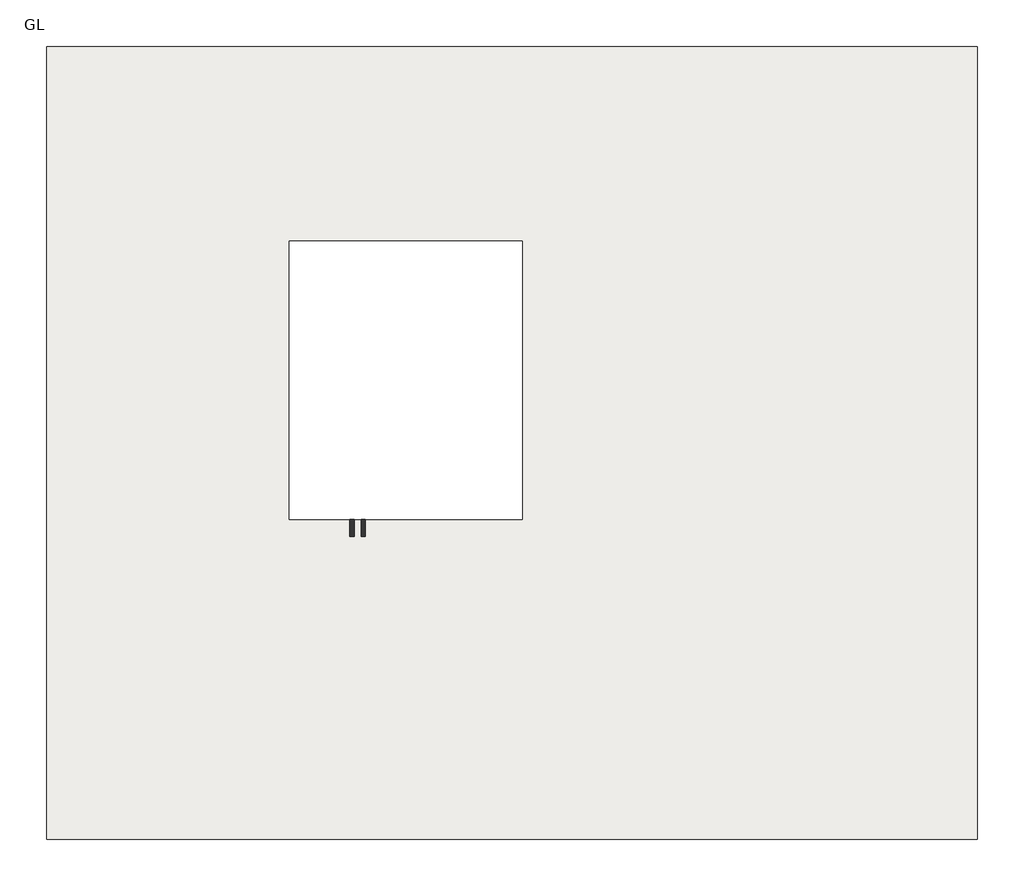
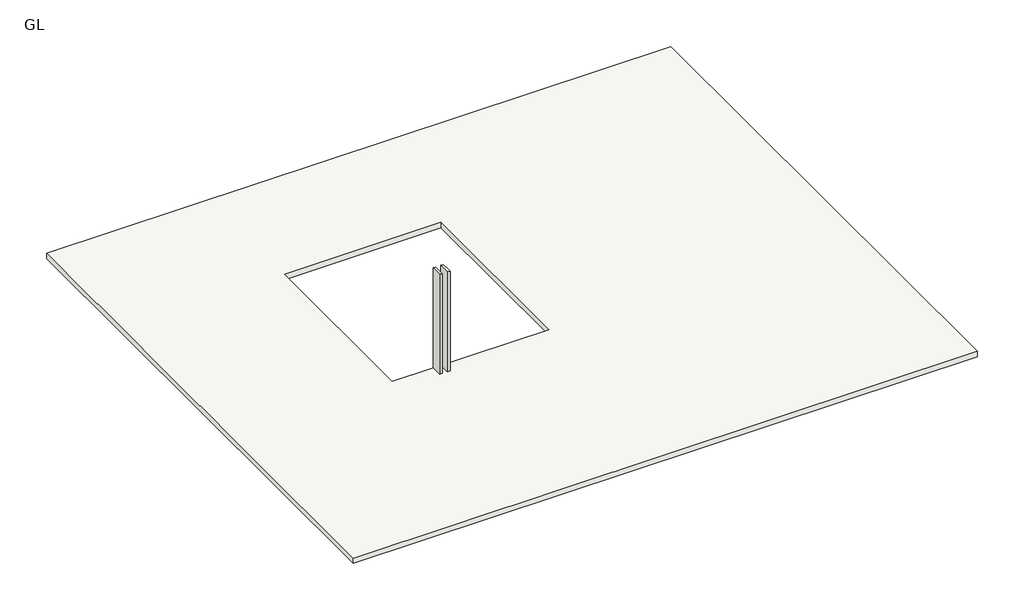
# One storey: 2 walls, 1 slab.
"""IFC4 building model written with IfcOpenShell, lengths in millimetres."""

from ifc_helpers import new_model, si_unit, frame, origin, place, context, project, spatial, polyline, outline, extrude, faceted_brep, element, save

model = new_model("IFC4")

# Units and contexts
model_context = context("Model", 3, world=origin())
ifc_project = project(units=[si_unit("LENGTHUNIT", "METRE", prefix="MILLI")], contexts=[model_context])

# Site, building, storey
site = spatial("IfcSite", under=ifc_project)
building = spatial("IfcBuilding", under=site)
storey = spatial("IfcBuildingStorey", under=building, Name="GL", Elevation=-304.8)

# Slab
placement = place(None, origin())
element("IfcSlab", 1, ObjectType="6\"", at=placement, inside=storey, context=model_context, shape_type="SweptSolid", body=[
    extrude(outline(polyline([(32209.0101634, 17689.5631811), (32209.0101634, -25287.2368189), (-18235.3898366, -25287.2368189), (-18235.3898366, 17689.5631811), (32209.0101634, 17689.5631811)]), holes=[polyline([(7553.0590234, 7136.1703059), (-5084.2350579, 7136.1703059), (-5084.2350579, -7961.058484), (7553.0590234, -7961.058484), (7553.0590234, 7136.1703059)])]), frame((0.0, 0.0, -762.0), z_axis=(0.0, 0.0, 1.0), x_axis=(1.0, 0.0, 0.0)), (0.0, 0.0, 1.0), 457.2),
])

# Walls
element("IfcWall", 2, ObjectType="9\"", at=placement, inside=storey, context=model_context, shape_type="Brep", body=[
    faceted_brep([(-1183.1942549, -7961.058484, -304.8), (-1183.1942549, -8875.458484, -304.8), (-1183.1942549, -8875.458484, 8229.6), (-1183.1942549, -7961.058484, 8229.6), (-954.5942549, -7961.058484, -304.8), (-954.5942549, -7961.058484, 8229.6), (-954.5942549, -8646.858484, 8229.6), (-954.5942549, -8875.458484, 8229.6), (-954.5942549, -8875.458484, 6858.0), (-954.5942549, -8875.458484, -304.8)], [[[0, 1, 2, 3]], [[4, 5, 6, 7, 8, 9]], [[1, 0, 4, 9]], [[3, 2, 7, 6, 5]], [[0, 3, 5, 4]], [[2, 1, 9, 8, 7]]]),
])
element("IfcWall", 3, ObjectType="9\"", at=placement, inside=storey, context=model_context, shape_type="SweptSolid", body=[
    extrude(outline(polyline([(-1792.7942549, -8875.458484), (-1792.7942549, -7961.058484), (-1564.1942549, -7961.058484), (-1564.1942549, -8875.458484), (-1792.7942549, -8875.458484)])), frame((0.0, 0.0, -304.8), z_axis=(0.0, 0.0, 1.0), x_axis=(1.0, 0.0, 0.0)), (0.0, 0.0, 1.0), 8534.4),
])

save(model, "model.ifc")

# Revit data of these elements
# Type "6\""
#   Assembly Code = "B1010"
#   Function = 0
#   Layers, outside or top first: 1' - 6" no material (function 1)
# Type "9\""
#   Assembly Code = "B2010"
#   Layers, outside or top first: 0' - 9" no material (function 1)
# Element 1 (IfcSlab, "6\"")
#   Height Offset From Level = 0' - 0"
#   Phase Created = New Construction
#   Materials on its faces: "Default Floor"
# Elements 2, 3 (IfcWall, "9\"")
#   Top Offset = 0' - 0"
#   Base Offset = 0' - 0"
#   Unconnected Height = 28' - 0"
#   wall height = 28' - 0"
#   Phase Created = New Construction
#   Base Constraint = GL
#   Materials on its faces: "st wall", "Default Wall"
# Materials
#   "Default Floor": colour RGB 128 128 128, transparency 0, Cost = 0
#   "st wall": class "Generic", colour RGB 85 49 28, transparency 0, Cost = 0
#   "Default Wall": colour RGB 128 128 128, transparency 0, Cost = 0
